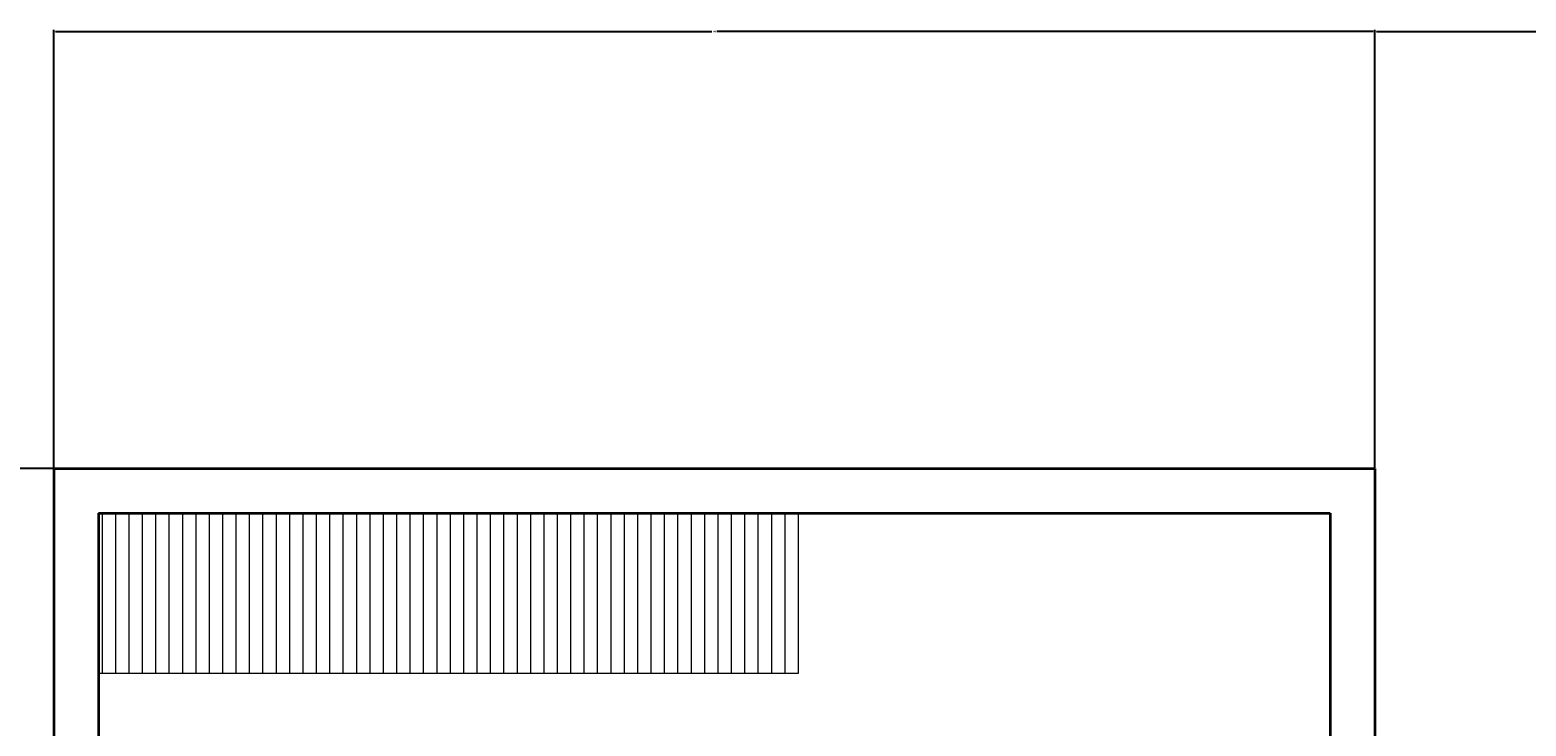
# Model space of a CAD drawing. Units: inches. Extents: x 3731 to 4318, y 1310 to 2388.
# Tile 40 of 57: x 3833 to 4000, y 2310 to 2388. Entities that reach past the tile are written whole.
import ezdxf

# ---------------------------------------------------------------- set-up
doc = ezdxf.new("R2010")
doc.units = ezdxf.units.IN
for name, color, linetype, lineweight in [('A-ANNO-DIMS', 2, 'Continuous', 18), ('A-FLOR-PATT', 252, 'Continuous', 13), ('A-WALL', 7, 'Continuous', 35)]:
    doc.layers.add(name, color=color, linetype=linetype, lineweight=lineweight)
doc.styles.get("Standard").update_dxf_attribs({"font": 'arial.ttf'})
doc.dimstyles.get("Standard").update_dxf_attribs({"dimtxt": 0.18, "dimasz": 0.18, "dimexe": 0.18, "dimexo": 0.0625, "dimgap": 0.09, "dimtad": 0, "dimtih": 1, "dimtoh": 1, "dimdec": 4, "dimzin": 0, "dimdsep": 46, "dimtxsty": 'Standard', "dimcen": 0.09, "dimadec": 0, "dimazin": 0, "dimtfac": 1, "dimtdec": 4, "dimtofl": 0, "dimtmove": 0, "dimatfit": 3, "dimfxl": 1, "dimtolj": 1, "dimtzin": 0, "dimarcsym": 0})

# ---------------------------------------------------------------- blocks, each defined once
blk = doc.blocks.new('*U1')
blk.add_line((0, -18), (0, 0))
blk = doc.blocks.new('*U2')
at = {"layer": 'A-FLOR-PATT', "color": 0, "linetype": 'ByBlock', "lineweight": -2, "transparency": 16777216, "rotation": 180}
for p in [(3840.6, 2315.38), (3842.1, 2315.38), (3843.6, 2315.38), (3845.1, 2315.38), (3846.6, 2315.38), (3848.1, 2315.38), (3849.6, 2315.38), (3851.1, 2315.38), (3852.6, 2315.38), (3854.1, 2315.38), (3855.6, 2315.38), (3857.1, 2315.38), (3858.6, 2315.38), (3860.1, 2315.38), (3861.6, 2315.38), (3863.1, 2315.38), (3864.6, 2315.38), (3866.1, 2315.38), (3867.6, 2315.38), (3869.1, 2315.38), (3870.6, 2315.38), (3872.1, 2315.38), (3873.6, 2315.38), (3875.1, 2315.38), (3876.6, 2315.38), (3878.1, 2315.38), (3879.6, 2315.38), (3881.1, 2315.38), (3882.6, 2315.38), (3884.1, 2315.38), (3885.6, 2315.38), (3887.1, 2315.38), (3888.6, 2315.38), (3890.1, 2315.38), (3891.6, 2315.38), (3893.1, 2315.38), (3894.6, 2315.38), (3896.1, 2315.38), (3897.6, 2315.38), (3899.1, 2315.38), (3900.6, 2315.38), (3902.1, 2315.38), (3903.6, 2315.38), (3905.1, 2315.38), (3906.6, 2315.38), (3908.1, 2315.38), (3909.6, 2315.38), (3911.1, 2315.38), (3912.6, 2315.38), (3914.1, 2315.38), (3915.6, 2315.38), (3917.1, 2315.38), (3918.6, 2315.38)]:
    blk.add_blockref('*U1', p, dxfattribs=at)
blk = doc.blocks.new('*D33')
at = {"layer": 'A-ANNO-DIMS', "color": 0, "lineweight": -2, "transparency": 16777216}
for p, q in [((3835.15, 2338.38), (3731.41, 2338.38)), ((3731.59, 2338.2), (3731.59, 1849.06)), ((3731.59, 1359.56), (3731.59, 1848.7)), ((3835.15, 1359.38), (3731.41, 1359.38))]:
    blk.add_line(p, q, dxfattribs=at)
at = {"layer": 'A-ANNO-DIMS', "color": 0, "transparency": 16777216}
for points in [[(3731.56, 2338.2), (3731.62, 2338.2), (3731.59, 2338.38)], [(3731.56, 1359.56), (3731.62, 1359.56), (3731.59, 1359.38)]]:
    blk.add_solid(points, dxfattribs=at)
at = {"layer": 'Defpoints', "color": 0, "transparency": 16777216}
for p in [(3731.59, 2338.38), (3835.21, 2338.38), (3835.21, 1359.38)]:
    blk.add_point(p, dxfattribs=at)
at = {"layer": 'A-ANNO-DIMS', "color": 0, "transparency": 16777216, "insert": (3731.59, 1848.88), "char_height": 0.18, "attachment_point": 5}
blk.add_mtext('\\A1;979', dxfattribs=at)
blk = doc.blocks.new('*D34')
at = {"layer": 'A-ANNO-DIMS', "color": 0, "lineweight": -2, "transparency": 16777216}
for p, q in [((3835.21, 2338.44), (3835.21, 2387.51)), ((3835.39, 2387.33), (3908.93, 2387.33)), ((3983.03, 2387.33), (3909.49, 2387.33)), ((3983.21, 2338.44), (3983.21, 2387.51))]:
    blk.add_line(p, q, dxfattribs=at)
at = {"layer": 'A-ANNO-DIMS', "color": 0, "transparency": 16777216}
for points in [[(3835.39, 2387.36), (3835.39, 2387.3), (3835.21, 2387.33)], [(3983.03, 2387.36), (3983.03, 2387.3), (3983.21, 2387.33)]]:
    blk.add_solid(points, dxfattribs=at)
at = {"layer": 'Defpoints', "color": 0, "transparency": 16777216}
for p in [(3983.21, 2387.33), (3835.21, 2338.38), (3983.21, 2338.38)]:
    blk.add_point(p, dxfattribs=at)
at = {"layer": 'A-ANNO-DIMS', "color": 0, "transparency": 16777216, "insert": (3909.21, 2387.33), "char_height": 0.18, "attachment_point": 5}
blk.add_mtext('\\A1;148', dxfattribs=at)
blk = doc.blocks.new('*D35')
at = {"layer": 'A-ANNO-DIMS', "color": 0, "lineweight": -2, "transparency": 16777216}
for p, q in [((3983.21, 2338.44), (3983.21, 2387.51)), ((3983.39, 2387.33), (4042.93, 2387.33)), ((4103.03, 2387.33), (4043.49, 2387.33)), ((4103.21, 2338.44), (4103.21, 2387.51))]:
    blk.add_line(p, q, dxfattribs=at)
at = {"layer": 'A-ANNO-DIMS', "color": 0, "transparency": 16777216}
for points in [[(3983.39, 2387.36), (3983.39, 2387.3), (3983.21, 2387.33)], [(4103.03, 2387.36), (4103.03, 2387.3), (4103.21, 2387.33)]]:
    blk.add_solid(points, dxfattribs=at)
at = {"layer": 'Defpoints', "color": 0, "transparency": 16777216}
for p in [(4103.21, 2387.33), (3983.21, 2338.38), (4103.21, 2338.38)]:
    blk.add_point(p, dxfattribs=at)
at = {"layer": 'A-ANNO-DIMS', "color": 0, "transparency": 16777216, "insert": (4043.21, 2387.33), "char_height": 0.18, "attachment_point": 5}
blk.add_mtext('\\A1;120', dxfattribs=at)

msp = doc.modelspace()

# ---------------------------------------------------------------- linework, layer by layer
at = {"layer": 'A-FLOR-PATT'}
msp.add_line((3918.6, 2315.38), (3840.21, 2315.38), dxfattribs=at)
at = {"layer": 'A-WALL'}
for p, q in [((3835.21, 2338.38), (3835.21, 1359.38)), ((3835.21, 2338.38), (3983.21, 2338.38)), ((3983.21, 2338.38), (3983.21, 2262.38)), ((3840.21, 2333.38), (3840.21, 2156.38)), ((3840.21, 2333.38), (3978.21, 2333.38)), ((3978.21, 2333.38), (3978.21, 2223.38))]:
    msp.add_line(p, q, dxfattribs=at)

# ---------------------------------------------------------------- block references
at = {"layer": 'A-FLOR-PATT'}
msp.add_blockref('*U2', (0, 0), dxfattribs=at)

# ---------------------------------------------------------------- dimensions: what is measured, and where the dimension line sits
at = {"layer": 'A-ANNO-DIMS'}
for base, p1, p2, picture, middle in [((3983.21, 2387.33), (3835.21, 2338.38), (3983.21, 2338.38), '*D34', (3909.21, 2387.33)), ((4103.21, 2387.33), (3983.21, 2338.38), (4103.21, 2338.38), '*D35', (4043.21, 2387.33))]:
    dim = msp.add_linear_dim(base=base, p1=p1, p2=p2, dimstyle='Standard', override={"dimdec": 0, "dimlfac": 1, "dimrnd": 0, "dimzin": 0, "dimdsep": 46, "dimlunit": 2}, dxfattribs=at)
    dim.commit()
    dim.dimension.update_dxf_attribs({"geometry": picture, "text_midpoint": middle})
dim = msp.add_linear_dim(base=(3731.59, 2338.38), p1=(3835.21, 1359.38), p2=(3835.21, 2338.38), angle=90, dimstyle='Standard', override={"dimdec": 0, "dimlfac": 1, "dimrnd": 0, "dimzin": 0, "dimdsep": 46, "dimlunit": 2}, dxfattribs=at)
dim.commit()
dim.dimension.update_dxf_attribs({"geometry": '*D33', "text_midpoint": (3731.59, 1848.88)})

doc.saveas('drawing.dxf')
